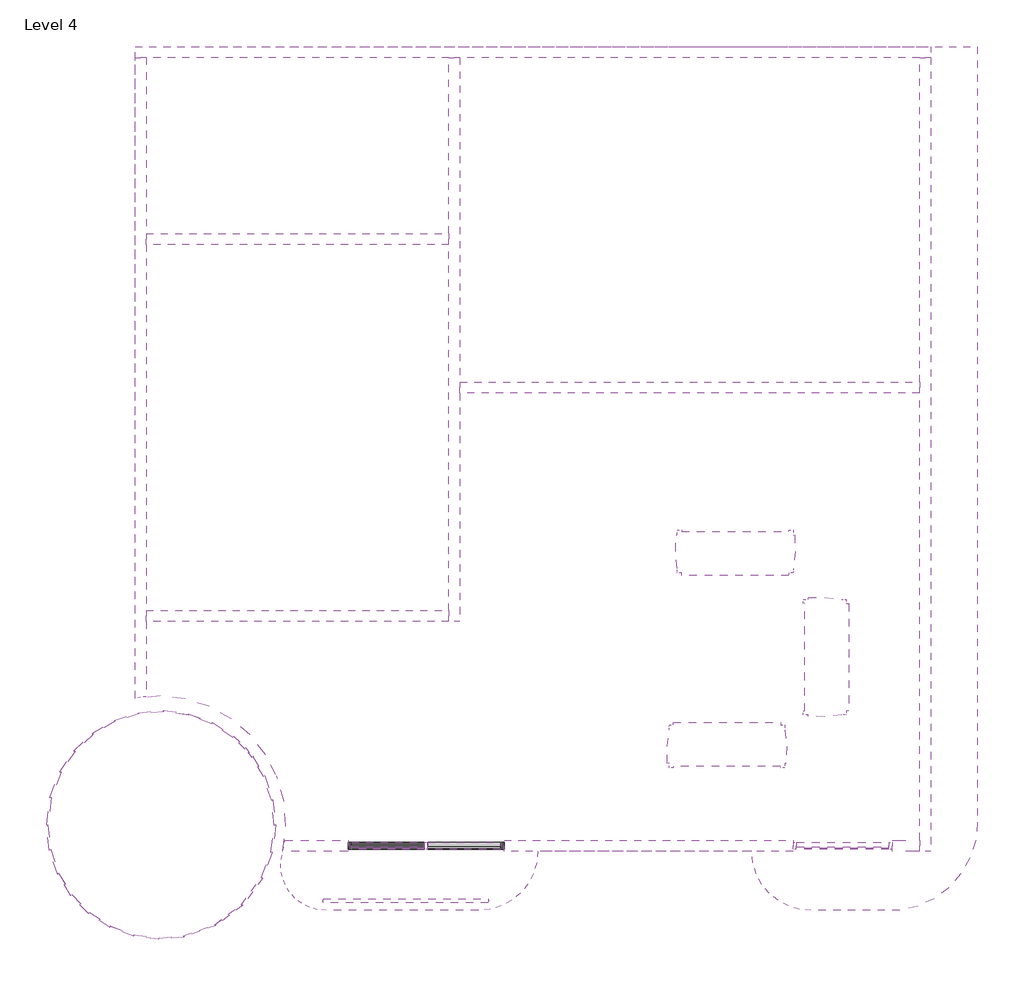
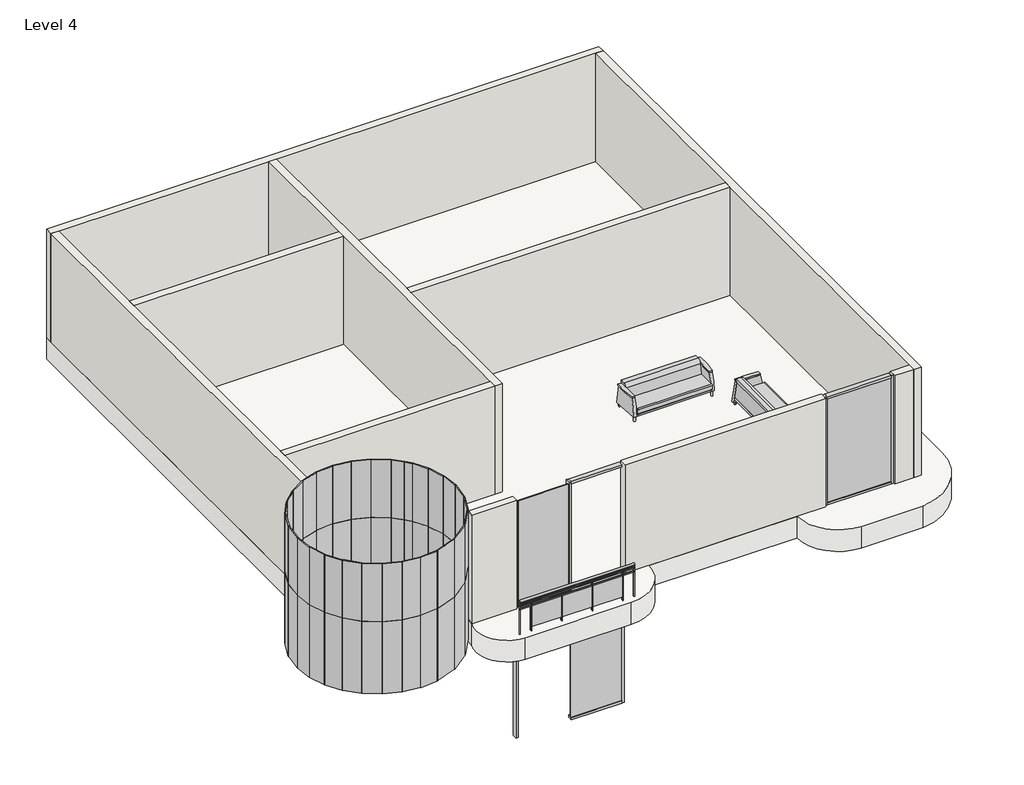
# One storey, incomplete: 59 plates, 11 members, 10 walls, 3 furniture elements, 1 railing, 1 slab.
"""IFC4 building model written with IfcOpenShell, lengths in millimetres."""

from ifc_helpers import new_model, si_unit, point, frame, frame_2d, origin, place, context, project, spatial, polyline, circle_curve, ellipse_curve, trimmed, segment, composite_curve, outline, extrude, faceted_brep, transform, mapped, element, save
from ifc_brep_helpers import plane_surface, revolved_surface, extruded_surface, advanced_brep
from components import furniture_aff9b2fb, member_eaba9652, member_3f395ae9, member_0c868e12, member_7bc42366, system_panel_glazed_f1c144f9, system_panel_glazed_8ed2b2ee, system_panel_glazed_c7815b78, system_panel_glazed_220ba5f3, system_panel_glazed_11fb153e, system_panel_glazed_2f540b85, system_panel_glazed_4848e608, system_panel_glazed_8b35a0ff, system_panel_glazed_87282c25, system_panel_glazed_6d1bb68c, system_panel_glazed_cb3ffd69, system_panel_glazed_404d015f, system_panel_glazed_7b556abe, system_panel_glazed_370bf902

model = new_model("IFC4")

# Units and contexts
model_context = context("Model", 3, world=origin())
ifc_project = project(units=[si_unit("LENGTHUNIT", "METRE", prefix="MILLI")], contexts=[model_context])

# Site, building, storey
site = spatial("IfcSite", under=ifc_project)
building = spatial("IfcBuilding", under=site)
storey = spatial("IfcBuildingStorey", under=building, Name="Level 4", Elevation=9144.0)

# Furniture
placement = place(None, origin())
furniture_shape = furniture_aff9b2fb(model_context)
element("IfcFurniture", 1, ObjectType="Sofa-Pensi : 84\"", at=placement, inside=storey, context=model_context, shape_type="MappedRepresentation", body=[
    mapped(furniture_shape, transform((-2244.8524991, 3650.1964615, 10972.8), x_axis=(1.0, 0.0, 0.0), y_axis=(0.0, 1.0, 0.0), z_axis=(0.0, 0.0, 1.0))),
])
element("IfcFurniture", 2, ObjectType="Sofa-Pensi : 84\"", at=placement, inside=storey, context=model_context, shape_type="MappedRepresentation", body=[
    mapped(furniture_shape, transform((-12.736413, 1720.492712, 10972.8), x_axis=(0.0, 1.0, 0.0), y_axis=(-1.0, 0.0, 0.0), z_axis=(0.0, 0.0, 1.0))),
])
element("IfcFurniture", 3, ObjectType="Sofa-Pensi : 84\"", at=placement, inside=storey, context=model_context, shape_type="MappedRepresentation", body=[
    mapped(furniture_shape, transform((-1840.0399991, 648.4161336, 10972.8), x_axis=(-1.0, 0.0, 0.0), y_axis=(0.0, -1.0, 0.0), z_axis=(0.0, 0.0, 1.0))),
])

# Members
member_shape = member_eaba9652(model_context)
element("IfcMember", 4, ObjectType="Rectangular Mullion : 2.5\" x 5\" rectangular", at=placement, inside=storey, context=model_context, shape_type="MappedRepresentation", body=[
    mapped(member_shape, transform((-7672.5789001, -1482.8937024, 10972.8), x_axis=(-1.0, 0.0, 0.0), y_axis=(0.0, 1.0, 0.0), z_axis=(0.0, 0.0, -1.0))),
])
member_2_shape = member_3f395ae9(model_context)
element("IfcMember", 5, ObjectType="Rectangular Mullion : 2.5\" x 5\" rectangular", at=placement, inside=storey, context=model_context, shape_type="MappedRepresentation", body=[
    mapped(member_2_shape, transform((-9111.7115512, -1482.8937024, 7315.2), x_axis=(-1.0, 0.0, 0.0), y_axis=(0.0, 1.0, 0.0), z_axis=(0.0, 0.0, -1.0))),
])
element("IfcMember", 6, ObjectType="Rectangular Mullion : 2.5\" x 5\" rectangular", at=placement, inside=storey, context=model_context, shape_type="MappedRepresentation", body=[
    mapped(member_2_shape, transform((-899.4462491, -1482.8937024, 10972.8), x_axis=(-1.0, 0.0, 0.0), y_axis=(0.0, 1.0, 0.0), z_axis=(0.0, 0.0, -1.0))),
])
element("IfcMember", 7, ObjectType="Rectangular Mullion : 2.5\" x 5\" rectangular", at=placement, inside=storey, context=model_context, shape_type="MappedRepresentation", body=[
    mapped(member_2_shape, transform((-6233.4462491, -1482.8937024, 10363.2), x_axis=(1.0, 0.0, 0.0), y_axis=(0.0, 1.0, 0.0), z_axis=(0.0, 0.0, 1.0))),
])
element("IfcMember", 8, ObjectType="Rectangular Mullion : 2.5\" x 5\" rectangular", at=placement, inside=storey, context=model_context, shape_type="MappedRepresentation", body=[
    mapped(member_2_shape, transform((929.3537509, -1482.8937024, 14020.8), x_axis=(1.0, 0.0, 0.0), y_axis=(0.0, 1.0, 0.0), z_axis=(0.0, 0.0, 1.0))),
])
member_3_shape = member_0c868e12(model_context)
element("IfcMember", 9, ObjectType="Rectangular Mullion : 2.5\" x 5\" rectangular", at=placement, inside=storey, context=model_context, shape_type="MappedRepresentation", body=[
    mapped(member_3_shape, transform((-9048.2115512, -1482.8937024, 10363.2), x_axis=(0.0, 0.0, 1.0), y_axis=(0.0, 1.0, 0.0), z_axis=(-1.0, 0.0, 0.0))),
])
element("IfcMember", 10, ObjectType="Rectangular Mullion : 2.5\" x 5\" rectangular", at=placement, inside=storey, context=model_context, shape_type="MappedRepresentation", body=[
    mapped(member_3_shape, transform((-7640.8289001, -1482.8937024, 14020.8), x_axis=(0.0, 0.0, 1.0), y_axis=(0.0, 1.0, 0.0), z_axis=(-1.0, 0.0, 0.0))),
])
element("IfcMember", 11, ObjectType="Rectangular Mullion : 2.5\" x 5\" rectangular", at=placement, inside=storey, context=model_context, shape_type="MappedRepresentation", body=[
    mapped(member_3_shape, transform((-6296.9462491, -1482.8937024, 7315.2), x_axis=(0.0, 0.0, -1.0), y_axis=(0.0, 1.0, 0.0), z_axis=(1.0, 0.0, 0.0))),
])
element("IfcMember", 12, ObjectType="Rectangular Mullion : 2.5\" x 5\" rectangular", at=placement, inside=storey, context=model_context, shape_type="MappedRepresentation", body=[
    mapped(member_3_shape, transform((-7704.3289001, -1482.8937024, 10972.8), x_axis=(0.0, 0.0, -1.0), y_axis=(0.0, 1.0, 0.0), z_axis=(1.0, 0.0, 0.0))),
])
member_4_shape = member_7bc42366(model_context)
element("IfcMember", 13, ObjectType="Rectangular Mullion : 2.5\" x 5\" rectangular", at=placement, inside=storey, context=model_context, shape_type="MappedRepresentation", body=[
    mapped(member_4_shape, transform((-835.9462491, -1482.8937024, 14020.8), x_axis=(0.0, 0.0, 1.0), y_axis=(0.0, 1.0, 0.0), z_axis=(-1.0, 0.0, 0.0))),
])
element("IfcMember", 14, ObjectType="Rectangular Mullion : 2.5\" x 5\" rectangular", at=placement, inside=storey, context=model_context, shape_type="MappedRepresentation", body=[
    mapped(member_4_shape, transform((865.8537509, -1482.8937024, 10972.8), x_axis=(0.0, 0.0, -1.0), y_axis=(0.0, 1.0, 0.0), z_axis=(1.0, 0.0, 0.0))),
])

# Plates
system_panel_glazed_shape = system_panel_glazed_f1c144f9(model_context)
element("IfcPlate", 15, ObjectType="System Panel : Glazed", at=placement, inside=storey, context=model_context, shape_type="MappedRepresentation", body=[
    mapped(system_panel_glazed_shape, transform((-14541.9245022, -346.5978939, 10972.8), x_axis=(-0.3551689475306269, -0.9348021281051873, 0.0), y_axis=(0.9348021281051873, -0.3551689475306269, 0.0), z_axis=(0.0, 0.0, 1.0))),
])
element("IfcPlate", 16, ObjectType="System Panel : Glazed", at=placement, inside=storey, context=model_context, shape_type="MappedRepresentation", body=[
    mapped(system_panel_glazed_shape, transform((-10582.1178502, -1851.0877948, 10972.8), x_axis=(0.35516894753064066, 0.934802128105182, 0.0), y_axis=(-0.934802128105182, 0.35516894753064066, 0.0), z_axis=(0.0, 0.0, 1.0))),
])
element("IfcPlate", 17, ObjectType="System Panel : Glazed", at=placement, inside=storey, context=model_context, shape_type="MappedRepresentation", body=[
    mapped(system_panel_glazed_shape, transform((-10459.5232171, -1354.5613954, 10972.8), x_axis=(0.12073632210407237, 0.9926846128175765, 0.0), y_axis=(-0.9926846128175765, 0.12073632210407237, 0.0), z_axis=(0.0, 0.0, 1.0))),
])
element("IfcPlate", 18, ObjectType="System Panel : Glazed", at=placement, inside=storey, context=model_context, shape_type="MappedRepresentation", body=[
    mapped(system_panel_glazed_shape, transform((-14664.5191354, -843.1242933, 10972.8), x_axis=(-0.12073632210406239, -0.9926846128175777, 0.0), y_axis=(0.9926846128175777, -0.12073632210406239, 0.0), z_axis=(0.0, 0.0, 1.0))),
])
system_panel_glazed_2_shape = system_panel_glazed_8ed2b2ee(model_context)
element("IfcPlate", 19, ObjectType="System Panel : Glazed", at=placement, inside=storey, context=model_context, shape_type="MappedRepresentation", body=[
    mapped(system_panel_glazed_2_shape, transform((-11841.3777431, -3082.3793017, 10972.8), x_axis=(0.9398911711666007, 0.3414741371803665, 0.0), y_axis=(-0.3414741371803665, 0.9398911711666007, 0.0), z_axis=(0.0, 0.0, 1.0))),
])
element("IfcPlate", 20, ObjectType="System Panel : Glazed", at=placement, inside=storey, context=model_context, shape_type="MappedRepresentation", body=[
    mapped(system_panel_glazed_2_shape, transform((-10858.9635423, -2345.1728692, 10972.8), x_axis=(0.5905687200141164, 0.8069873524045393, 0.0), y_axis=(-0.8069873524045393, 0.5905687200141164, 0.0), z_axis=(0.0, 0.0, 1.0))),
])
element("IfcPlate", 21, ObjectType="System Panel : Glazed", at=placement, inside=storey, context=model_context, shape_type="MappedRepresentation", body=[
    mapped(system_panel_glazed_2_shape, transform((-11295.3522982, -2786.8279712, 10972.8), x_axis=(0.7998453025525061, 0.6002062078858317, 0.0), y_axis=(-0.6002062078858317, 0.7998453025525061, 0.0), z_axis=(0.0, 0.0, 1.0))),
])
system_panel_glazed_3_shape = system_panel_glazed_c7815b78(model_context)
element("IfcPlate", 22, ObjectType="System Panel : Glazed", at=placement, inside=storey, context=model_context, shape_type="MappedRepresentation", body=[
    mapped(system_panel_glazed_3_shape, transform((-10454.4737362, -864.5204039, 10972.8), x_axis=(-0.11050163420416614, 0.993875942378227, 0.0), y_axis=(-0.993875942378227, -0.11050163420416614, 0.0), z_axis=(0.0, 0.0, 1.0))),
])
element("IfcPlate", 23, ObjectType="System Panel : Glazed", at=placement, inside=storey, context=model_context, shape_type="MappedRepresentation", body=[
    mapped(system_panel_glazed_3_shape, transform((-14669.5686163, -1333.1652848, 10972.8), x_axis=(0.11050163420415136, -0.9938759423782286, 0.0), y_axis=(0.9938759423782286, 0.11050163420415136, 0.0), z_axis=(0.0, 0.0, 1.0))),
])
element("IfcPlate", 24, ObjectType="System Panel : Glazed", at=placement, inside=storey, context=model_context, shape_type="MappedRepresentation", body=[
    mapped(system_panel_glazed_3_shape, transform((-11410.1424167, 681.5611944, 10972.8), x_axis=(-0.8396018558176894, 0.5432022861766066, 0.0), y_axis=(-0.5432022861766066, -0.8396018558176894, 0.0), z_axis=(0.0, 0.0, 1.0))),
])
element("IfcPlate", 25, ObjectType="System Panel : Glazed", at=placement, inside=storey, context=model_context, shape_type="MappedRepresentation", body=[
    mapped(system_panel_glazed_3_shape, transform((-13212.0893695, 919.590846, 10972.8), x_axis=(-0.9518517343814786, -0.3065587639506839, 0.0), y_axis=(0.3065587639506839, -0.9518517343814786, 0.0), z_axis=(0.0, 0.0, 1.0))),
])
element("IfcPlate", 26, ObjectType="System Panel : Glazed", at=placement, inside=storey, context=model_context, shape_type="MappedRepresentation", body=[
    mapped(system_panel_glazed_3_shape, transform((-12839.7224363, -3201.1142893, 10972.8), x_axis=(0.9913878918151698, -0.1309581916577702, 0.0), y_axis=(0.1309581916577702, 0.9913878918151698, 0.0), z_axis=(0.0, 0.0, 1.0))),
])
element("IfcPlate", 27, ObjectType="System Panel : Glazed", at=placement, inside=storey, context=model_context, shape_type="MappedRepresentation", body=[
    mapped(system_panel_glazed_3_shape, transform((-14365.783041, -2213.7896382, 10972.8), x_axis=(0.5257859322352114, -0.8506169252157811, 0.0), y_axis=(0.8506169252157811, 0.5257859322352114, 0.0), z_axis=(0.0, 0.0, 1.0))),
])
element("IfcPlate", 28, ObjectType="System Panel : Glazed", at=placement, inside=storey, context=model_context, shape_type="MappedRepresentation", body=[
    mapped(system_panel_glazed_3_shape, transform((-13713.8999358, -2879.2468831, 10972.8), x_axis=(0.8396018558176805, -0.5432022861766201, 0.0), y_axis=(0.5432022861766201, 0.8396018558176805, 0.0), z_axis=(0.0, 0.0, 1.0))),
])
element("IfcPlate", 29, ObjectType="System Panel : Glazed", at=placement, inside=storey, context=model_context, shape_type="MappedRepresentation", body=[
    mapped(system_panel_glazed_3_shape, transform((-14014.4059364, 446.2272921, 10972.8), x_axis=(-0.7286232370002992, -0.6849147235263715, 0.0), y_axis=(0.6849147235263715, -0.7286232370002992, 0.0), z_axis=(0.0, 0.0, 1.0))),
])
element("IfcPlate", 30, ObjectType="System Panel : Glazed", at=placement, inside=storey, context=model_context, shape_type="MappedRepresentation", body=[
    mapped(system_panel_glazed_3_shape, transform((-12284.3199161, 1003.4286006, 10972.8), x_axis=(-0.9913878918151723, 0.13095819165775144, 0.0), y_axis=(-0.13095819165775144, -0.9913878918151723, 0.0), z_axis=(0.0, 0.0, 1.0))),
])
element("IfcPlate", 31, ObjectType="System Panel : Glazed", at=placement, inside=storey, context=model_context, shape_type="MappedRepresentation", body=[
    mapped(system_panel_glazed_3_shape, transform((-12752.8652893, 1013.0855973, 10972.8), x_axis=(-0.9959419324521102, -0.08999815100076568, 0.0), y_axis=(0.08999815100076568, -0.9959419324521102, 0.0), z_axis=(0.0, 0.0, 1.0))),
])
element("IfcPlate", 32, ObjectType="System Panel : Glazed", at=placement, inside=storey, context=model_context, shape_type="MappedRepresentation", body=[
    mapped(system_panel_glazed_3_shape, transform((-11829.3381514, 891.0915272, 10972.8), x_axis=(-0.9384120429483949, 0.3455182160891376, 0.0), y_axis=(-0.3455182160891376, -0.9384120429483949, 0.0), z_axis=(0.0, 0.0, 1.0))),
])
element("IfcPlate", 33, ObjectType="System Panel : Glazed", at=placement, inside=storey, context=model_context, shape_type="MappedRepresentation", body=[
    mapped(system_panel_glazed_3_shape, transform((-10557.4115054, -407.3204039, 10972.8), x_axis=(-0.3261077326604367, 0.9453326116764772, 0.0), y_axis=(-0.9453326116764772, -0.3261077326604367, 0.0), z_axis=(0.0, 0.0, 1.0))),
])
element("IfcPlate", 34, ObjectType="System Panel : Glazed", at=placement, inside=storey, context=model_context, shape_type="MappedRepresentation", body=[
    mapped(system_panel_glazed_3_shape, transform((-12371.1770631, -3210.771286, 10972.8), x_axis=(0.9959419324521115, 0.08999815100075001, 0.0), y_axis=(-0.08999815100075001, 0.9959419324521115, 0.0), z_axis=(0.0, 0.0, 1.0))),
])
element("IfcPlate", 35, ObjectType="System Panel : Glazed", at=placement, inside=storey, context=model_context, shape_type="MappedRepresentation", body=[
    mapped(system_panel_glazed_3_shape, transform((-13294.7042011, -3088.7772159, 10972.8), x_axis=(0.9384120429483891, -0.34551821608915334, 0.0), y_axis=(0.34551821608915334, 0.9384120429483891, 0.0), z_axis=(0.0, 0.0, 1.0))),
])
element("IfcPlate", 36, ObjectType="System Panel : Glazed", at=placement, inside=storey, context=model_context, shape_type="MappedRepresentation", body=[
    mapped(system_panel_glazed_3_shape, transform((-14076.8350959, -2582.7572647, 10972.8), x_axis=(0.6997834615185511, -0.7143550286692988, 0.0), y_axis=(0.7143550286692988, 0.6997834615185511, 0.0), z_axis=(0.0, 0.0, 1.0))),
])
element("IfcPlate", 37, ObjectType="System Panel : Glazed", at=placement, inside=storey, context=model_context, shape_type="MappedRepresentation", body=[
    mapped(system_panel_glazed_3_shape, transform((-14566.6308471, -1790.3652848, 10972.8), x_axis=(0.32610773266042153, -0.9453326116764824, 0.0), y_axis=(0.9453326116764824, 0.32610773266042153, 0.0), z_axis=(0.0, 0.0, 1.0))),
])
element("IfcPlate", 38, ObjectType="System Panel : Glazed", at=placement, inside=storey, context=model_context, shape_type="MappedRepresentation", body=[
    mapped(system_panel_glazed_3_shape, transform((-14318.3113206, 89.4787227, 10972.8), x_axis=(-0.5603879632167612, -0.8282302401396425, 0.0), y_axis=(0.8282302401396425, -0.5603879632167612, 0.0), z_axis=(0.0, 0.0, 1.0))),
])
element("IfcPlate", 39, ObjectType="System Panel : Glazed", at=placement, inside=storey, context=model_context, shape_type="MappedRepresentation", body=[
    mapped(system_panel_glazed_3_shape, transform((-13639.5625299, 727.5108588, 10972.8), x_axis=(-0.8612707706620224, -0.5081462974412448, 0.0), y_axis=(0.5081462974412448, -0.8612707706620224, 0.0), z_axis=(0.0, 0.0, 1.0))),
])
system_panel_glazed_4_shape = system_panel_glazed_220ba5f3(model_context)
element("IfcPlate", 40, ObjectType="System Panel : Glazed", at=placement, inside=storey, context=model_context, shape_type="MappedRepresentation", body=[
    mapped(system_panel_glazed_4_shape, transform((-10742.3305673, -4.7597883, 10972.8), x_axis=(-0.5152811917631037, 0.8570211744263939, 0.0), y_axis=(-0.8570211744263939, -0.5152811917631037, 0.0), z_axis=(0.0, 0.0, 1.0))),
])
system_panel_glazed_5_shape = system_panel_glazed_11fb153e(model_context)
element("IfcPlate", 41, ObjectType="System Panel : Glazed", at=placement, inside=storey, context=model_context, shape_type="MappedRepresentation", body=[
    mapped(system_panel_glazed_5_shape, transform((-11098.0043985, 445.2241463, 10972.8), x_axis=(-0.7256671855033587, 0.6880458821064435, 0.0), y_axis=(-0.6880458821064435, -0.7256671855033587, 0.0), z_axis=(0.0, 0.0, 1.0))),
])
system_panel_glazed_6_shape = system_panel_glazed_2f540b85(model_context)
element("IfcPlate", 42, ObjectType="System Panel : Glazed", at=placement, inside=storey, context=model_context, shape_type="MappedRepresentation", body=[
    mapped(system_panel_glazed_6_shape, transform((-10917.0903061, 255.9395759, 10972.8), x_axis=(-0.6357445726375757, 0.7718995001694627, 0.0), y_axis=(-0.7718995001694627, -0.6357445726375757, 0.0), z_axis=(0.0, 0.0, 1.0))),
])
system_panel_glazed_7_shape = system_panel_glazed_4848e608(model_context)
element("IfcPlate", 43, ObjectType="System Panel : Glazed", at=placement, inside=storey, context=model_context, shape_type="MappedRepresentation", body=[
    mapped(system_panel_glazed_7_shape, transform((-14669.5686163, -1333.1652848, 13004.8), x_axis=(0.11050163420415136, -0.9938759423782286, 0.0), y_axis=(0.9938759423782286, 0.11050163420415136, 0.0), z_axis=(0.0, 0.0, 1.0))),
])
element("IfcPlate", 44, ObjectType="System Panel : Glazed", at=placement, inside=storey, context=model_context, shape_type="MappedRepresentation", body=[
    mapped(system_panel_glazed_7_shape, transform((-14365.783041, -2213.7896382, 13004.8), x_axis=(0.5257859322352114, -0.8506169252157811, 0.0), y_axis=(0.8506169252157811, 0.5257859322352114, 0.0), z_axis=(0.0, 0.0, 1.0))),
])
element("IfcPlate", 45, ObjectType="System Panel : Glazed", at=placement, inside=storey, context=model_context, shape_type="MappedRepresentation", body=[
    mapped(system_panel_glazed_7_shape, transform((-13713.8999358, -2879.2468831, 13004.8), x_axis=(0.8396018558176805, -0.5432022861766201, 0.0), y_axis=(0.5432022861766201, 0.8396018558176805, 0.0), z_axis=(0.0, 0.0, 1.0))),
])
element("IfcPlate", 46, ObjectType="System Panel : Glazed", at=placement, inside=storey, context=model_context, shape_type="MappedRepresentation", body=[
    mapped(system_panel_glazed_7_shape, transform((-12839.7224363, -3201.1142893, 13004.8), x_axis=(0.9913878918151698, -0.13095819165777017, 0.0), y_axis=(0.13095819165777017, 0.9913878918151698, 0.0), z_axis=(0.0, 0.0, 1.0))),
])
element("IfcPlate", 47, ObjectType="System Panel : Glazed", at=placement, inside=storey, context=model_context, shape_type="MappedRepresentation", body=[
    mapped(system_panel_glazed_7_shape, transform((-12371.1770631, -3210.771286, 13004.8), x_axis=(0.9959419324521115, 0.08999815100075001, 0.0), y_axis=(-0.08999815100075001, 0.9959419324521115, 0.0), z_axis=(0.0, 0.0, 1.0))),
])
element("IfcPlate", 48, ObjectType="System Panel : Glazed", at=placement, inside=storey, context=model_context, shape_type="MappedRepresentation", body=[
    mapped(system_panel_glazed_7_shape, transform((-13294.7042011, -3088.7772159, 13004.8), x_axis=(0.9384120429483891, -0.34551821608915334, 0.0), y_axis=(0.34551821608915334, 0.9384120429483891, 0.0), z_axis=(0.0, 0.0, 1.0))),
])
element("IfcPlate", 49, ObjectType="System Panel : Glazed", at=placement, inside=storey, context=model_context, shape_type="MappedRepresentation", body=[
    mapped(system_panel_glazed_7_shape, transform((-14076.8350959, -2582.7572647, 13004.8), x_axis=(0.6997834615185511, -0.7143550286692988, 0.0), y_axis=(0.7143550286692988, 0.6997834615185511, 0.0), z_axis=(0.0, 0.0, 1.0))),
])
element("IfcPlate", 50, ObjectType="System Panel : Glazed", at=placement, inside=storey, context=model_context, shape_type="MappedRepresentation", body=[
    mapped(system_panel_glazed_7_shape, transform((-14566.6308471, -1790.3652848, 13004.8), x_axis=(0.32610773266042153, -0.9453326116764824, 0.0), y_axis=(0.9453326116764824, 0.32610773266042153, 0.0), z_axis=(0.0, 0.0, 1.0))),
])
element("IfcPlate", 51, ObjectType="System Panel : Glazed", at=placement, inside=storey, context=model_context, shape_type="MappedRepresentation", body=[
    mapped(system_panel_glazed_7_shape, transform((-10454.4737362, -864.5204039, 13004.8), x_axis=(-0.11050163420416614, 0.993875942378227, 0.0), y_axis=(-0.993875942378227, -0.11050163420416614, 0.0), z_axis=(0.0, 0.0, 1.0))),
])
element("IfcPlate", 52, ObjectType="System Panel : Glazed", at=placement, inside=storey, context=model_context, shape_type="MappedRepresentation", body=[
    mapped(system_panel_glazed_7_shape, transform((-10557.4115054, -407.3204039, 13004.8), x_axis=(-0.3261077326604368, 0.9453326116764772, 0.0), y_axis=(-0.9453326116764772, -0.3261077326604368, 0.0), z_axis=(0.0, 0.0, 1.0))),
])
element("IfcPlate", 53, ObjectType="System Panel : Glazed", at=placement, inside=storey, context=model_context, shape_type="MappedRepresentation", body=[
    mapped(system_panel_glazed_7_shape, transform((-11410.1424167, 681.5611944, 13004.8), x_axis=(-0.8396018558176894, 0.5432022861766066, 0.0), y_axis=(-0.5432022861766066, -0.8396018558176894, 0.0), z_axis=(0.0, 0.0, 1.0))),
])
element("IfcPlate", 54, ObjectType="System Panel : Glazed", at=placement, inside=storey, context=model_context, shape_type="MappedRepresentation", body=[
    mapped(system_panel_glazed_7_shape, transform((-11829.3381514, 891.0915272, 13004.8), x_axis=(-0.9384120429483949, 0.3455182160891376, 0.0), y_axis=(-0.3455182160891376, -0.9384120429483949, 0.0), z_axis=(0.0, 0.0, 1.0))),
])
element("IfcPlate", 55, ObjectType="System Panel : Glazed", at=placement, inside=storey, context=model_context, shape_type="MappedRepresentation", body=[
    mapped(system_panel_glazed_7_shape, transform((-12284.3199161, 1003.4286006, 13004.8), x_axis=(-0.9913878918151723, 0.1309581916577514, 0.0), y_axis=(-0.1309581916577514, -0.9913878918151723, 0.0), z_axis=(0.0, 0.0, 1.0))),
])
element("IfcPlate", 56, ObjectType="System Panel : Glazed", at=placement, inside=storey, context=model_context, shape_type="MappedRepresentation", body=[
    mapped(system_panel_glazed_7_shape, transform((-12752.8652893, 1013.0855973, 13004.8), x_axis=(-0.9959419324521102, -0.08999815100076568, 0.0), y_axis=(0.08999815100076568, -0.9959419324521102, 0.0), z_axis=(0.0, 0.0, 1.0))),
])
element("IfcPlate", 57, ObjectType="System Panel : Glazed", at=placement, inside=storey, context=model_context, shape_type="MappedRepresentation", body=[
    mapped(system_panel_glazed_7_shape, transform((-13212.0893695, 919.590846, 13004.8), x_axis=(-0.9518517343814786, -0.3065587639506839, 0.0), y_axis=(0.3065587639506839, -0.9518517343814786, 0.0), z_axis=(0.0, 0.0, 1.0))),
])
element("IfcPlate", 58, ObjectType="System Panel : Glazed", at=placement, inside=storey, context=model_context, shape_type="MappedRepresentation", body=[
    mapped(system_panel_glazed_7_shape, transform((-13639.5625299, 727.5108588, 13004.8), x_axis=(-0.8612707706620223, -0.508146297441245, 0.0), y_axis=(0.508146297441245, -0.8612707706620223, 0.0), z_axis=(0.0, 0.0, 1.0))),
])
element("IfcPlate", 59, ObjectType="System Panel : Glazed", at=placement, inside=storey, context=model_context, shape_type="MappedRepresentation", body=[
    mapped(system_panel_glazed_7_shape, transform((-14014.4059364, 446.2272921, 13004.8), x_axis=(-0.7286232370002992, -0.6849147235263715, 0.0), y_axis=(0.6849147235263715, -0.7286232370002992, 0.0), z_axis=(0.0, 0.0, 1.0))),
])
element("IfcPlate", 60, ObjectType="System Panel : Glazed", at=placement, inside=storey, context=model_context, shape_type="MappedRepresentation", body=[
    mapped(system_panel_glazed_7_shape, transform((-14318.3113206, 89.4787227, 13004.8), x_axis=(-0.5603879632167612, -0.8282302401396425, 0.0), y_axis=(0.8282302401396425, -0.5603879632167612, 0.0), z_axis=(0.0, 0.0, 1.0))),
])
system_panel_glazed_8_shape = system_panel_glazed_8b35a0ff(model_context)
element("IfcPlate", 61, ObjectType="System Panel : Glazed", at=placement, inside=storey, context=model_context, shape_type="MappedRepresentation", body=[
    mapped(system_panel_glazed_8_shape, transform((-10742.3305673, -4.7597883, 13004.8), x_axis=(-0.5152811917631037, 0.8570211744263939, 0.0), y_axis=(-0.8570211744263939, -0.5152811917631037, 0.0), z_axis=(0.0, 0.0, 1.0))),
])
system_panel_glazed_9_shape = system_panel_glazed_87282c25(model_context)
element("IfcPlate", 62, ObjectType="System Panel : Glazed", at=placement, inside=storey, context=model_context, shape_type="MappedRepresentation", body=[
    mapped(system_panel_glazed_9_shape, transform((-10917.0903061, 255.9395759, 13004.8), x_axis=(-0.6357445726375757, 0.7718995001694627, 0.0), y_axis=(-0.7718995001694627, -0.6357445726375757, 0.0), z_axis=(0.0, 0.0, 1.0))),
])
system_panel_glazed_10_shape = system_panel_glazed_6d1bb68c(model_context)
element("IfcPlate", 63, ObjectType="System Panel : Glazed", at=placement, inside=storey, context=model_context, shape_type="MappedRepresentation", body=[
    mapped(system_panel_glazed_10_shape, transform((-11098.0043985, 445.2241463, 13004.8), x_axis=(-0.7256671855033587, 0.6880458821064435, 0.0), y_axis=(-0.6880458821064435, -0.7256671855033587, 0.0), z_axis=(0.0, 0.0, 1.0))),
])
system_panel_glazed_11_shape = system_panel_glazed_cb3ffd69(model_context)
element("IfcPlate", 64, ObjectType="System Panel : Glazed", at=placement, inside=storey, context=model_context, shape_type="MappedRepresentation", body=[
    mapped(system_panel_glazed_11_shape, transform((-10582.1178502, -1851.0877948, 13004.8), x_axis=(0.35516894753064066, 0.934802128105182, 0.0), y_axis=(-0.934802128105182, 0.35516894753064066, 0.0), z_axis=(0.0, 0.0, 1.0))),
])
element("IfcPlate", 65, ObjectType="System Panel : Glazed", at=placement, inside=storey, context=model_context, shape_type="MappedRepresentation", body=[
    mapped(system_panel_glazed_11_shape, transform((-10459.5232171, -1354.5613954, 13004.8), x_axis=(0.1207363221040724, 0.9926846128175765, 0.0), y_axis=(-0.9926846128175765, 0.1207363221040724, 0.0), z_axis=(0.0, 0.0, 1.0))),
])
element("IfcPlate", 66, ObjectType="System Panel : Glazed", at=placement, inside=storey, context=model_context, shape_type="MappedRepresentation", body=[
    mapped(system_panel_glazed_11_shape, transform((-14541.9245022, -346.5978939, 13004.8), x_axis=(-0.3551689475306269, -0.9348021281051873, 0.0), y_axis=(0.9348021281051873, -0.3551689475306269, 0.0), z_axis=(0.0, 0.0, 1.0))),
])
element("IfcPlate", 67, ObjectType="System Panel : Glazed", at=placement, inside=storey, context=model_context, shape_type="MappedRepresentation", body=[
    mapped(system_panel_glazed_11_shape, transform((-14664.5191354, -843.1242933, 13004.8), x_axis=(-0.1207363221040624, -0.9926846128175777, 0.0), y_axis=(0.9926846128175777, -0.1207363221040624, 0.0), z_axis=(0.0, 0.0, 1.0))),
])
system_panel_glazed_12_shape = system_panel_glazed_404d015f(model_context)
element("IfcPlate", 68, ObjectType="System Panel : Glazed", at=placement, inside=storey, context=model_context, shape_type="MappedRepresentation", body=[
    mapped(system_panel_glazed_12_shape, transform((-11841.3777431, -3082.3793017, 13004.8), x_axis=(0.9398911711666007, 0.3414741371803665, 0.0), y_axis=(-0.3414741371803665, 0.9398911711666007, 0.0), z_axis=(0.0, 0.0, 1.0))),
])
element("IfcPlate", 69, ObjectType="System Panel : Glazed", at=placement, inside=storey, context=model_context, shape_type="MappedRepresentation", body=[
    mapped(system_panel_glazed_12_shape, transform((-10858.9635423, -2345.1728692, 13004.8), x_axis=(0.5905687200141164, 0.8069873524045393, 0.0), y_axis=(-0.8069873524045393, 0.5905687200141164, 0.0), z_axis=(0.0, 0.0, 1.0))),
])
element("IfcPlate", 70, ObjectType="System Panel : Glazed", at=placement, inside=storey, context=model_context, shape_type="MappedRepresentation", body=[
    mapped(system_panel_glazed_12_shape, transform((-11295.3522982, -2786.8279712, 13004.8), x_axis=(0.7998453025525062, 0.6002062078858316, 0.0), y_axis=(-0.6002062078858316, 0.7998453025525062, 0.0), z_axis=(0.0, 0.0, 1.0))),
])
system_panel_glazed_13_shape = system_panel_glazed_7b556abe(model_context)
element("IfcPlate", 71, ObjectType="System Panel : Glazed", at=placement, inside=storey, context=model_context, shape_type="MappedRepresentation", body=[
    mapped(system_panel_glazed_13_shape, transform((-6968.8875746, -1482.8937024, 7378.7), x_axis=(-1.0, 0.0, 0.0), y_axis=(0.0, -1.0, 0.0), z_axis=(0.0, 0.0, 1.0))),
])
element("IfcPlate", 72, ObjectType="System Panel : Glazed", at=placement, inside=storey, context=model_context, shape_type="MappedRepresentation", body=[
    mapped(system_panel_glazed_13_shape, transform((-8376.2702257, -1482.8937024, 11036.3), x_axis=(-1.0, 0.0, 0.0), y_axis=(0.0, -1.0, 0.0), z_axis=(0.0, 0.0, 1.0))),
])
system_panel_glazed_14_shape = system_panel_glazed_370bf902(model_context)
element("IfcPlate", 73, ObjectType="System Panel : Glazed", at=placement, inside=storey, context=model_context, shape_type="MappedRepresentation", body=[
    mapped(system_panel_glazed_14_shape, transform((14.9537509, -1482.8937024, 11036.3), x_axis=(-1.0, 0.0, 0.0), y_axis=(0.0, -1.0, 0.0), z_axis=(0.0, 0.0, 1.0))),
])

# Railing
element("IfcRailing", 74, ObjectType="Glass Panel - Bottom Fill", at=placement, inside=storey, context=model_context, shape_type="SolidModel", body=[
    advanced_brep(
    [(-9570.3600838, -2460.0257683, 11887.2), (-9570.3600838, -2536.2257683, 11887.2), (-6522.3600838, -2460.0257683, 11887.2), (-6522.3600838, -2536.2257683, 11887.2)],
    [
        (0, 1, ellipse_curve(frame((-9570.3600838, -2498.1257683, 11887.2), z_axis=(-1.0, 0.0, 0.0), x_axis=(0.0, -1.0, 0.0)), 38.1, 28.575)),
        (1, 0, ellipse_curve(frame((-9570.3600838, -2498.1257683, 11887.2), z_axis=(-1.0, 0.0, 0.0), x_axis=(0.0, -1.0, 0.0)), 38.1, 28.575)),
        (2, 3, ellipse_curve(frame((-6522.3600838, -2498.1257683, 11887.2), z_axis=(1.0, 0.0, 0.0), x_axis=(0.0, -1.0, 0.0)), 38.1, 28.575)),
        (3, 2, ellipse_curve(frame((-6522.3600838, -2498.1257683, 11887.2), z_axis=(1.0, 0.0, 0.0), x_axis=(0.0, -1.0, 0.0)), 38.1, 28.575)),
        (0, 2),
        (3, 1),
    ],
    [
        plane_surface(frame((-9570.3600838, -2498.1257683, 11887.2), z_axis=(-1.0, 0.0, 0.0), x_axis=(0.0, 1.0, 0.0))),
        plane_surface(frame((-6522.3600838, -2498.1257683, 11887.2), z_axis=(1.0, 0.0, 0.0), x_axis=(0.0, 1.0, 0.0))),
        extruded_surface(trimmed(ellipse_curve(frame((-6522.3600838, -2498.1257683, 11887.2), z_axis=(-1.0, 0.0, 0.0), x_axis=(0.0, -1.0, 0.0)), 38.1, 28.575), [point((-6522.3600838, -2460.0257683, 11887.2))], [point((-6522.3600838, -2536.2257683, 11887.2))], True, "CARTESIAN"), (-3048.0, 0.0, 0.0), 3048.0),
        extruded_surface(trimmed(ellipse_curve(frame((-6522.3600838, -2498.1257683, 11887.2), z_axis=(-1.0, 0.0, 0.0), x_axis=(0.0, -1.0, 0.0)), 38.1, 28.575), [point((-6522.3600838, -2536.2257683, 11887.2))], [point((-6522.3600838, -2460.0257683, 11887.2))], True, "CARTESIAN"), (-3048.0, 0.0, 0.0), 3048.0),
    ],
    [
        (0, [[1, 2]]),
        (1, [[3, 4]]),
        (2, [[-1, 5, -4, 6]]),
        (3, [[-2, -6, -3, -5]]),
    ],
),
    extrude(outline(polyline([(-9570.3600838, -2510.8257683), (-9570.3600838, -2485.4257683), (-6522.3600838, -2485.4257683), (-6522.3600838, -2510.8257683), (-9570.3600838, -2510.8257683)])), frame((0.0, 0.0, 11772.9), z_axis=(0.0, 0.0, 1.0), x_axis=(1.0, 0.0, 0.0)), (0.0, 0.0, 1.0), 25.4),
    extrude(outline(polyline([(-9570.3600838, -2510.8257683), (-9570.3600838, -2485.4257683), (-6522.3600838, -2485.4257683), (-6522.3600838, -2510.8257683), (-9570.3600838, -2510.8257683)])), frame((0.0, 0.0, 11671.3), z_axis=(0.0, 0.0, 1.0), x_axis=(1.0, 0.0, 0.0)), (0.0, 0.0, 1.0), 25.4),
    extrude(outline(polyline([(-6833.5100838, -2523.5257683), (-6833.5100838, -2472.7257683), (-6820.8100838, -2472.7257683), (-6820.8100838, -2523.5257683), (-6833.5100838, -2523.5257683)])), frame((0.0, 0.0, 10972.8), z_axis=(0.0, 0.0, 1.0), x_axis=(1.0, 0.0, 0.0)), (0.0, 0.0, 1.0), 885.6788223),
    extrude(outline(polyline([(-7639.9600838, -2491.5906113), (-6827.1600838, -2491.5906113), (-6827.1600838, -2497.9406113), (-7639.9600838, -2497.9406113), (-7639.9600838, -2491.5906113)])), frame((0.0, 0.0, 11074.4), z_axis=(0.0, 0.0, 1.0), x_axis=(1.0, 0.0, 0.0)), (0.0, 0.0, 1.0), 596.9),
    extrude(outline(polyline([(-7646.3100838, -2523.5257683), (-7646.3100838, -2472.7257683), (-7633.6100838, -2472.7257683), (-7633.6100838, -2523.5257683), (-7646.3100838, -2523.5257683)])), frame((0.0, 0.0, 10972.8), z_axis=(0.0, 0.0, 1.0), x_axis=(1.0, 0.0, 0.0)), (0.0, 0.0, 1.0), 885.6788223),
    extrude(outline(polyline([(-8452.7600838, -2491.5906113), (-7639.9600838, -2491.5906113), (-7639.9600838, -2497.9406113), (-8452.7600838, -2497.9406113), (-8452.7600838, -2491.5906113)])), frame((0.0, 0.0, 11074.4), z_axis=(0.0, 0.0, 1.0), x_axis=(1.0, 0.0, 0.0)), (0.0, 0.0, 1.0), 596.9),
    extrude(outline(polyline([(-8459.1100838, -2523.5257683), (-8459.1100838, -2472.7257683), (-8446.4100838, -2472.7257683), (-8446.4100838, -2523.5257683), (-8459.1100838, -2523.5257683)])), frame((0.0, 0.0, 10972.8), z_axis=(0.0, 0.0, 1.0), x_axis=(1.0, 0.0, 0.0)), (0.0, 0.0, 1.0), 885.6788223),
    extrude(outline(polyline([(-9265.5600838, -2491.5906113), (-8452.7600838, -2491.5906113), (-8452.7600838, -2497.9406113), (-9265.5600838, -2497.9406113), (-9265.5600838, -2491.5906113)])), frame((0.0, 0.0, 11074.4), z_axis=(0.0, 0.0, 1.0), x_axis=(1.0, 0.0, 0.0)), (0.0, 0.0, 1.0), 596.9),
    extrude(outline(polyline([(-9271.9100838, -2523.5257683), (-9271.9100838, -2472.7257683), (-9259.2100838, -2472.7257683), (-9259.2100838, -2523.5257683), (-9271.9100838, -2523.5257683)])), frame((0.0, 0.0, 10972.8), z_axis=(0.0, 0.0, 1.0), x_axis=(1.0, 0.0, 0.0)), (0.0, 0.0, 1.0), 885.6788223),
    extrude(outline(polyline([(-6535.0600838, -2507.6507683), (-6535.0600838, -2488.6007683), (-6516.0100838, -2488.6007683), (-6516.0100838, -2507.6507683), (-6535.0600838, -2507.6507683)])), frame((0.0, 0.0, 10972.8), z_axis=(0.0, 0.0, 1.0), x_axis=(1.0, 0.0, 0.0)), (0.0, 0.0, 1.0), 885.6788223),
    extrude(outline(polyline([(-9576.7100838, -2507.6507683), (-9576.7100838, -2488.6007683), (-9557.6600838, -2488.6007683), (-9557.6600838, -2507.6507683), (-9576.7100838, -2507.6507683)])), frame((0.0, 0.0, 10972.8), z_axis=(0.0, 0.0, 1.0), x_axis=(1.0, 0.0, 0.0)), (0.0, 0.0, 1.0), 885.6788223),
])

# Slab
element("IfcSlab", 75, ObjectType="Generic - 2'", at=placement, inside=storey, context=model_context, shape_type="SweptSolid", body=[
    extrude(outline(composite_curve([segment(polyline([(2504.1537509, 13274.5062976), (2504.1537509, -1051.0937024)]), True, "CONTINUOUS"), segment(trimmed(circle_curve(frame_2d((865.9099456, -1051.0937024)), 1638.2438053), [point((2504.1537509, -1051.0937024))], [point((1069.0537509, -2676.6937024))], False, "CARTESIAN"), True, "CONTINUOUS"), segment(polyline([(1069.0537509, -2676.6937024), (-569.2462491, -2676.6937024)]), True, "CONTINUOUS"), segment(trimmed(circle_curve(frame_2d((-569.2462491, -1584.4937024)), 1092.2), [point((-569.2462491, -2676.6937024))], [point((-1661.4462491, -1584.4937024))], False, "CARTESIAN"), True, "CONTINUOUS"), segment(polyline([(-1661.4462491, -1584.4937024), (-5609.8647377, -1584.4937024)]), True, "CONTINUOUS"), segment(trimmed(circle_curve(frame_2d((-6702.0647377, -1584.4937024)), 1092.2), [point((-5609.8647377, -1584.4937024))], [point((-6702.0647377, -2676.6937024))], False, "CARTESIAN"), True, "CONTINUOUS"), segment(polyline([(-6702.0647377, -2676.6937024), (-9521.4647377, -2676.6937024)]), True, "CONTINUOUS"), segment(trimmed(circle_curve(frame_2d((-9521.4647377, -1843.8920375)), 832.801665), [point((-9521.4647377, -2676.6937024))], [point((-10312.8376694, -1584.4937024))], False, "CARTESIAN"), True, "CONTINUOUS"), segment(trimmed(circle_curve(frame_2d((-12612.6150686, -1075.1054509)), 2355.5153315), [point((-10312.8376694, -1584.4937024))], [point((-13040.6462491, 1241.1937063))], True, "CARTESIAN"), True, "CONTINUOUS"), segment(polyline([(-13040.6462491, 1241.1937063), (-13040.6462491, 13274.5062976), (2504.1537509, 13274.5062976)]), True, "CONTINUOUS")], self_intersect=False)), frame((0.0, 0.0, 10363.2), z_axis=(0.0, 0.0, 1.0), x_axis=(1.0, 0.0, 0.0)), (0.0, 0.0, 1.0), 609.6),
])

# Walls
element("IfcWall", 76, ObjectType="Generic - 8\"", at=placement, inside=storey, context=model_context, shape_type="Brep", body=[
    faceted_brep([(-13040.6462491, 13071.3062976, 10972.8), (-12837.4462491, 13071.3062976, 10972.8), (-7249.4462491, 13071.3062976, 10972.8), (-7046.2462491, 13071.3062976, 10972.8), (1437.3537509, 13071.3062976, 10972.8), (1640.5537509, 13071.3062976, 10972.8), (1640.5537509, 13071.3062976, 14020.8), (1437.3537509, 13071.3062976, 14020.8), (-7046.2462491, 13071.3062976, 14020.8), (-7249.4462491, 13071.3062976, 14020.8), (-12837.4462491, 13071.3062976, 14020.8), (-13040.6462491, 13071.3062976, 14020.8), (-13040.6462491, 13274.5062976, 10972.8), (-13040.6462491, 13274.5062976, 14020.8), (1640.5537509, 13274.5062976, 14020.8), (1640.5537509, 13274.5062976, 10972.8)], [[[0, 1, 2, 3, 4, 5, 6, 7, 8, 9, 10, 11]], [[12, 13, 14, 15]], [[5, 4, 3, 2, 1, 0, 12, 15]], [[11, 10, 9, 8, 7, 6, 14, 13]], [[6, 5, 15, 14]], [[0, 11, 13, 12]]]),
])
element("IfcWall", 77, ObjectType="Generic - 8\"", at=placement, inside=storey, context=model_context, shape_type="Brep", body=[
    faceted_brep([(1437.3537509, 13071.3062976, 10972.8), (1437.3537509, 7076.9062976, 10972.8), (1437.3537509, 6873.7062976, 10972.8), (1437.3537509, -1381.2937024, 10972.8), (1437.3537509, -1584.4937024, 10972.8), (1437.3537509, -1584.4937024, 14020.8), (1437.3537509, -1381.2937024, 14020.8), (1437.3537509, 6873.7062976, 14020.8), (1437.3537509, 7076.9062976, 14020.8), (1437.3537509, 13071.3062976, 14020.8), (1640.5537509, 13071.3062976, 10972.8), (1640.5537509, 13071.3062976, 14020.8), (1640.5537509, -1584.4937024, 14020.8), (1640.5537509, -1584.4937024, 10972.8)], [[[0, 1, 2, 3, 4, 5, 6, 7, 8, 9]], [[10, 11, 12, 13]], [[4, 3, 2, 1, 0, 10, 13]], [[9, 8, 7, 6, 5, 12, 11]], [[0, 9, 11, 10]], [[5, 4, 13, 12]]]),
])
element("IfcWall", 78, ObjectType="Generic - 8\"", at=placement, inside=storey, context=model_context, shape_type="AdvancedBrep", body=[
    advanced_brep(
    [(-13040.6462491, 13071.3062976, 10972.8), (-13040.6462491, 1241.1937063, 10972.8), (-13040.6462491, 1241.1937063, 14020.8), (-13040.6462491, 13071.3062976, 14020.8), (-12837.4462491, 13071.3062976, 10972.8), (-12837.4462491, 13071.3062976, 14020.8), (-12837.4462491, 9820.1062976, 14020.8), (-12837.4462491, 9616.9062976, 14020.8), (-12837.4462491, 2862.698962, 14020.8), (-12837.4462491, 2659.498962, 14020.8), (-12837.4462491, 1269.6553935, 14020.8), (-12837.4462491, 1269.6553935, 10972.8), (-12837.4462491, 2659.498962, 10972.8), (-12837.4462491, 2862.698962, 10972.8), (-12837.4462491, 9616.9062976, 10972.8), (-12837.4462491, 9820.1062976, 10972.8)],
    [
        (0, 1),
        (1, 2),
        (2, 3),
        (3, 0),
        (4, 5),
        (5, 6),
        (6, 7),
        (7, 8),
        (8, 9),
        (9, 10),
        (10, 11),
        (11, 12),
        (12, 13),
        (13, 14),
        (14, 15),
        (15, 4),
        (0, 4),
        (11, 1, circle_curve(frame((-12612.6150686, -1075.1054509, 10972.8), z_axis=(0.0, 0.0, 1.0), x_axis=(1.0, 0.0, 0.0)), 2355.5153315)),
        (2, 10, circle_curve(frame((-12612.6150686, -1075.1054509, 14020.8), z_axis=(0.0, 0.0, -1.0), x_axis=(1.0, 0.0, 0.0)), 2355.5153315)),
        (5, 3),
    ],
    [
        plane_surface(frame((-13040.6462491, 16068.5062976, 10972.8), z_axis=(-1.0, 0.0, 0.0), x_axis=(0.0, -1.0, 0.0))),
        plane_surface(frame((-12837.4462491, 16068.5062976, 10972.8), z_axis=(1.0, 0.0, 0.0), x_axis=(0.0, 1.0, 0.0))),
        plane_surface(frame((-13040.6462491, 13172.9062976, 10972.8), z_axis=(0.0, 0.0, -1.0), x_axis=(1.0, 0.0, 0.0))),
        plane_surface(frame((-13040.6462491, 1155.046339, 14020.8), z_axis=(0.0, 0.0, 1.0), x_axis=(1.0, 0.0, 0.0))),
        plane_surface(frame((-16139.4462491, 13071.3062976, 10972.8), z_axis=(0.0, 1.0, 0.0), x_axis=(1.0, 0.0, 0.0))),
        revolved_surface(polyline([(-10257.099737100001, -1075.1054509, 14020.8), (-10257.099737100001, -1075.1054509, 10972.8)]), (-12612.6150686, -1075.1054509, 10972.8), (0.0, 0.0, 1.0)),
    ],
    [
        (0, [[1, 2, 3, 4]]),
        (1, [[5, 6, 7, 8, 9, 10, 11, 12, 13, 14, 15, 16]]),
        (2, [[-1, 17, -16, -15, -14, -13, -12, 18]]),
        (3, [[-3, 19, -10, -9, -8, -7, -6, 20]]),
        (4, [[-4, -20, -5, -17]]),
        (5, [[-2, -18, -11, -19]]),
    ],
),
])
element("IfcWall", 79, ObjectType="Generic - 8\"", at=placement, inside=storey, context=model_context, shape_type="Brep", body=[
    faceted_brep([(-7249.4462491, 13071.3062976, 10972.8), (-7249.4462491, 9820.1062976, 10972.8), (-7249.4462491, 9616.9062976, 10972.8), (-7249.4462491, 2862.698962, 10972.8), (-7249.4462491, 2659.498962, 10972.8), (-7249.4462491, 2659.498962, 14020.8), (-7249.4462491, 2862.698962, 14020.8), (-7249.4462491, 9616.9062976, 14020.8), (-7249.4462491, 9820.1062976, 14020.8), (-7249.4462491, 13071.3062976, 14020.8), (-7046.2462491, 13071.3062976, 10972.8), (-7046.2462491, 13071.3062976, 14020.8), (-7046.2462491, 7076.9062976, 14020.8), (-7046.2462491, 6873.7062976, 14020.8), (-7046.2462491, 2659.498962, 14020.8), (-7046.2462491, 2659.498962, 10972.8), (-7046.2462491, 6873.7062976, 10972.8), (-7046.2462491, 7076.9062976, 10972.8)], [[[0, 1, 2, 3, 4, 5, 6, 7, 8, 9]], [[10, 11, 12, 13, 14, 15, 16, 17]], [[4, 3, 2, 1, 0, 10, 17, 16, 15]], [[9, 8, 7, 6, 5, 14, 13, 12, 11]], [[0, 9, 11, 10]], [[5, 4, 15, 14]]]),
])
element("IfcWall", 80, ObjectType="Generic - 8\"", at=placement, inside=storey, context=model_context, shape_type="SweptSolid", body=[
    extrude(outline(polyline([(1437.3537509, 6873.7062976), (-7046.2462491, 6873.7062976), (-7046.2462491, 7076.9062976), (1437.3537509, 7076.9062976), (1437.3537509, 6873.7062976)])), frame((0.0, 0.0, 10972.8), z_axis=(0.0, 0.0, 1.0), x_axis=(1.0, 0.0, 0.0)), (0.0, 0.0, 1.0), 3048.0),
])
element("IfcWall", 81, ObjectType="Generic - 8\"", at=placement, inside=storey, context=model_context, shape_type="SweptSolid", body=[
    extrude(outline(polyline([(-12837.4462491, 9820.1062976), (-7249.4462491, 9820.1062976), (-7249.4462491, 9616.9062976), (-12837.4462491, 9616.9062976), (-12837.4462491, 9820.1062976)])), frame((0.0, 0.0, 10972.8), z_axis=(0.0, 0.0, 1.0), x_axis=(1.0, 0.0, 0.0)), (0.0, 0.0, 1.0), 3048.0),
])
element("IfcWall", 82, ObjectType="Generic - 8\"", at=placement, inside=storey, context=model_context, shape_type="SweptSolid", body=[
    extrude(outline(polyline([(-12837.4462491, 2862.698962), (-7249.4462491, 2862.698962), (-7249.4462491, 2659.498962), (-12837.4462491, 2659.498962), (-12837.4462491, 2862.698962)])), frame((0.0, 0.0, 10972.8), z_axis=(0.0, 0.0, 1.0), x_axis=(1.0, 0.0, 0.0)), (0.0, 0.0, 1.0), 3048.0),
])
element("IfcWall", 83, ObjectType="Generic - 8\"", at=placement, inside=storey, context=model_context, shape_type="SweptSolid", body=[
    extrude(outline(composite_curve([segment(polyline([(-9111.7115512, -1584.4937024), (-10312.8376694, -1584.4937024)]), True, "CONTINUOUS"), segment(trimmed(circle_curve(frame_2d((-12612.6150686, -1075.1054509)), 2355.5153315), [point((-10312.8376694, -1584.4937024))], [point((-10277.0848865, -1381.2937024))], True, "CARTESIAN"), True, "CONTINUOUS"), segment(polyline([(-10277.0848865, -1381.2937024), (-9111.7115512, -1381.2937024), (-9111.7115512, -1584.4937024)]), True, "CONTINUOUS")], self_intersect=False)), frame((0.0, 0.0, 10972.8), z_axis=(0.0, 0.0, 1.0), x_axis=(1.0, 0.0, 0.0)), (0.0, 0.0, 1.0), 3048.0),
])
element("IfcWall", 84, ObjectType="Generic - 8\"", at=placement, inside=storey, context=model_context, shape_type="SweptSolid", body=[
    extrude(outline(polyline([(-899.4462491, -1584.4937024), (-6233.4462491, -1584.4937024), (-6233.4462491, -1381.2937024), (-899.4462491, -1381.2937024), (-899.4462491, -1584.4937024)])), frame((0.0, 0.0, 10972.8), z_axis=(0.0, 0.0, 1.0), x_axis=(1.0, 0.0, 0.0)), (0.0, 0.0, 1.0), 3048.0),
])
element("IfcWall", 85, ObjectType="Generic - 8\"", at=placement, inside=storey, context=model_context, shape_type="SweptSolid", body=[
    extrude(outline(polyline([(929.3537509, -1381.2937024), (1437.3537509, -1381.2937024), (1437.3537509, -1584.4937024), (929.3537509, -1584.4937024), (929.3537509, -1381.2937024)])), frame((0.0, 0.0, 10972.8), z_axis=(0.0, 0.0, 1.0), x_axis=(1.0, 0.0, 0.0)), (0.0, 0.0, 1.0), 3048.0),
])

save(model, "model.ifc")

# Revit data of these elements
# Type "Sofa-Pensi : 84\""
#   Assembly Code = "E2020200"
#   Length = 7' - 0"
#   Frame Material = Cherry
#   Seat Material = Linen, Beige
#   Feet Material = Steel, Chrome Plated
#   Default Elevation = 0
# Type "Rectangular Mullion : 2.5\" x 5\" rectangular"
#   built-in parameter 1007304 = 0.416667 (stored number, unit not read)
#   built-in parameter 1007301 = 0.104167 (stored number, unit not read)
#   built-in parameter 1007300 = 0.104167 (stored number, unit not read)
# Type "System Panel : Glazed"
#   Construction Type Id = "GSP4R"
#   Analytic Construction = "1/8 in Pilkington single glazing"
#   Visual Light Transmittance = 0.9
#   Solar Heat Gain Coefficient = 0.86
#   Heat Transfer Coefficient (U) = 1.18115 BTU/(h·ft²·°F)
# Type "Glass Panel - Bottom Fill"
#   Assembly Code = "C2010400"
#   built-in parameter 1008612 = 0.0416667 (stored number, unit not read)
#   built-in parameter 1008611 = 0.0416667 (stored number, unit not read)
#   built-in parameter 1008609 = 0.333333 (stored number, unit not read)
#   built-in parameter 1008604 = 0.166667 (stored number, unit not read)
#   built-in parameter 1008603 = 0.166667 (stored number, unit not read)
#   Railing Height = 3' - 0"
#   built-in parameter 1008630 = 2
#   built-in parameter 1008610 = 2
#   built-in parameter 1008618 = Baluster - Square : 3/4"
# Type "Generic - 2'"
#   Assembly Code = "B1010"
#   Function = 0
#   Layers, outside or top first: 2' - 0" no material (function 1)
# Type "Generic - 8\""
#   Assembly Code = "B2010"
#   Layers, outside or top first: 0' - 8" no material (function 1)
# Elements 1, 2, 3 (IfcFurniture, "Sofa-Pensi : 84\"")
#   Phase Created = New Construction
#   Materials on its faces: "Cherry", "Linen, Beige", "Steel, Chrome Plated"
# Elements 4, 5, 6, 7, 8, 9, 10, 11, 12, 13, 14 (IfcMember, "Rectangular Mullion : 2.5\" x 5\" rectangular")
#   Phase Created = New Construction
#   Materials on its faces: "Iron, Ductile"
# Elements 15, 16, 17, 18, 19, 20, 21, 22, 23, 24, 25, 26, 27, 28, 29, 30, 31, 32, 33, 34, 35, 36, 37, 38, 39, 40, 41, 42, 43, 44, 45, 46, 47, 48, 49, 50, 51, 52, 53, 54, 55, 56, 57, 58, 59, 60, 61, 62, 63, 64, 65, 66, 67, 68, 69, 70, 71, 72, 73 (IfcPlate, "System Panel : Glazed")
#   Phase Created = New Construction
#   Materials on its faces: "Glass"
# Element 74 (IfcRailing, "Glass Panel - Bottom Fill")
#   built-in parameter 1008621 = 6 (stored number, unit not read)
#   Phase Created = New Construction
#   Materials on its faces: "Glass"
# Element 75 (IfcSlab, "Generic - 2'")
#   Height Offset From Level = 6' - 0"
#   Phase Created = New Construction
#   Materials on its faces: "Default Floor"
# Elements 76, 77, 78, 79, 80, 81, 82, 83, 84, 85 (IfcWall, "Generic - 8\"")
#   built-in parameter 1001111 = 6' - 0"
#   Top Offset = 0' - 0"
#   Base Offset = 6' - 0"
#   Unconnected Height = 10' - 0"
#   wall height = 10' - 0"
#   Phase Created = New Construction
#   Base Constraint = Level 4
#   Materials on its faces: "Default Wall"
# Materials
#   "Cherry": class "Wood", colour RGB 226 177 128, transparency 0, Description = "Prunus Serotina", Cost = 0
#   "Linen, Beige": class "Textile", colour RGB 249 239 230, transparency 0, Description = "Linen, beige", Cost = 0
#   "Steel, Chrome Plated": class "Metal", colour RGB 17 17 17, transparency 0, Description = "Chromiuim plated steel", Cost = 0
#   "Iron, Ductile": class "Metal", colour RGB 0 0 0, transparency 0, Description = "Ductile cast iron", Cost = 0
#   "Glass": class "Glass", colour RGB 0 128 192, transparency 0.75, Description = "Soda Lime Glass", Cost = 0
#   "Default Floor": colour RGB 128 128 128, transparency 0
#   "Default Wall": colour RGB 128 128 128, transparency 0
